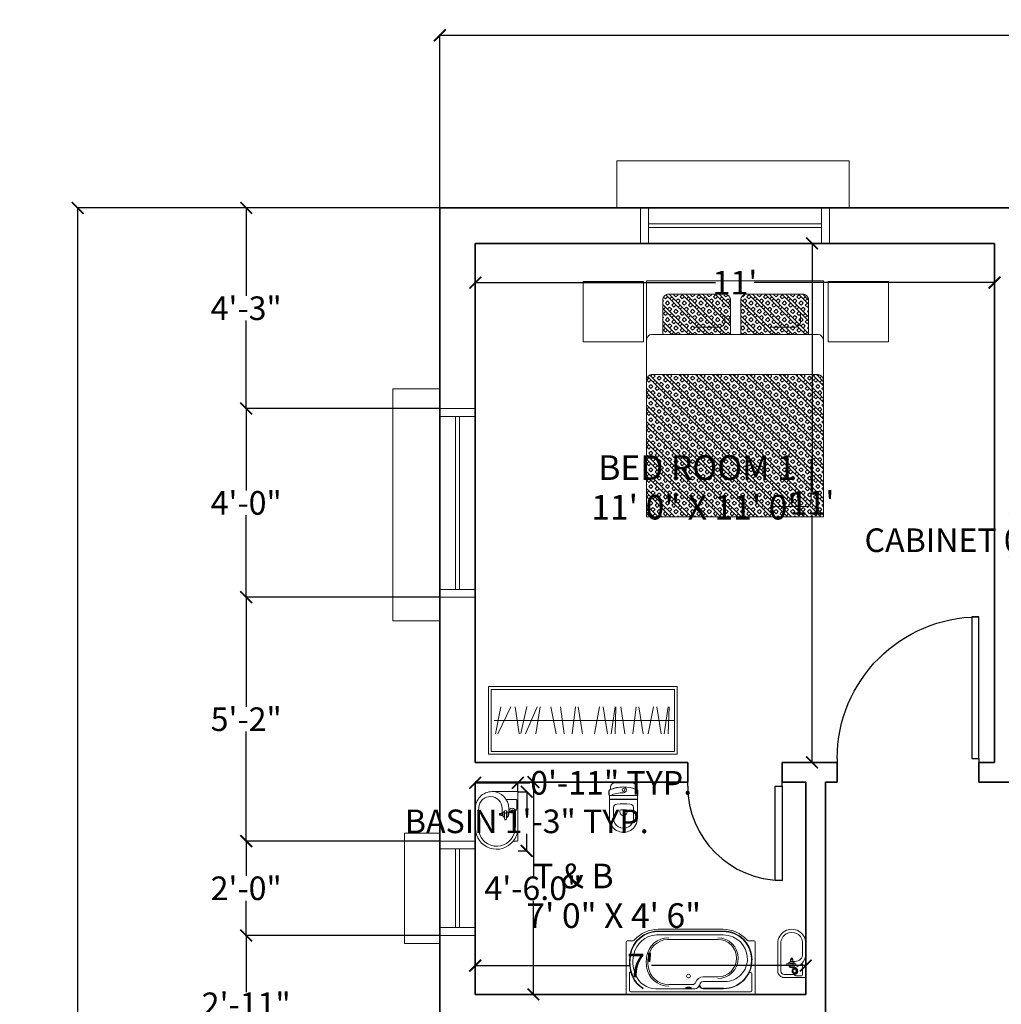
# Model space of a CAD drawing. Units: inches. Extents: x 844 to 2234, y 346 to 1084.
# Tile 49 of 93: x 1590 to 1840, y 828 to 1078. Entities that reach past the tile are written whole.
import ezdxf

# ---------------------------------------------------------------- set-up
doc = ezdxf.new("R2010")
doc.units = ezdxf.units.IN
doc.header["$MEASUREMENT"] = 0
for name, color, linetype, lineweight in [('A-ANNO-DIMS', 2, 'Continuous', 18), ('A-AREA-IDEN', 7, 'Continuous', 18), ('A-FLOR-FIXT', 8, 'Continuous', 18), ('A-WALL', 7, 'Continuous', 35), ('beds', 130, 'Continuous', 18), ('doors', 170, 'Continuous', 25), ('furniture', 8, 'Continuous', 18), ('windows', 1, 'Continuous', 18)]:
    doc.layers.add(name, color=color, linetype=linetype, lineweight=lineweight)
doc.styles.get("Standard").update_dxf_attribs({"font": 'arial.ttf'})
doc.dimstyles.get("Standard").update_dxf_attribs({"dimtxt": 6, "dimasz": 3, "dimexe": 0.18, "dimexo": 0.0625, "dimgap": 0.09, "dimtad": 0, "dimtih": 1, "dimtoh": 1, "dimdec": 1, "dimzin": 0, "dimdsep": 46, "dimlunit": 3, "dimtxsty": 'Standard', "dimblk": 'ARCHTICK', "dimcen": 0.09, "dimadec": 0, "dimazin": 0, "dimtfac": 1, "dimtdec": 1, "dimtofl": 0, "dimtmove": 0, "dimatfit": 3, "dimfxl": 1, "dimtolj": 1, "dimtzin": 0, "dimarcsym": 0})
pattern_1 = [(135, (-1377.70473, -125.71507), (-0.070710678, -0.070710678), []), (135, (-1377.68705, -125.69739), (-0.070710678, -0.070710678), []), (45, (-1377.70473, -125.71507), (-0.070710678, 0.070710678), [-0.025, 0.025]), (45, (-1377.72241, -125.69739), (-0.070710678, 0.070710678), [-0.025, 0.025]), (45, (-1377.74009, -125.67972), (-0.070710678, 0.070710678), [0.025, -0.025]), (45, (-1377.75776, -125.66204), (-0.070710678, 0.070710678), [0.025, -0.025]), (135, (-1377.66938, -125.67972), (-0.070710678, -0.070710678), [0.025, -0.025]), (135, (-1377.6517, -125.66204), (-0.070710678, -0.070710678), [0.025, -0.025])]

# ---------------------------------------------------------------- blocks, each defined once
blk = doc.blocks.new('*U2')
for p, q in [((0, 0), (0, -6)), ((36, 0), (36, -6))]:
    blk.add_line(p, q)
blk.add_lwpolyline([(0, 0), (0, 36), (1.75, 36), (1.75, 0)], close=True)
blk.add_arc((0, 0), 36, 0, 90)
blk = doc.blocks.new('*U4')
for p, q in [((0, 0), (0, -6)), ((24, 0), (24, -6))]:
    blk.add_line(p, q)
blk.add_lwpolyline([(0, 0), (0, 24), (1.75, 24), (1.75, 0)], close=True)
blk.add_arc((0, 0), 24, 0, 90)
blk = doc.blocks.new('MAT-P10')
h = blk.add_hatch()
h.set_pattern_fill('BOX', color=256, scale=0.1, angle=45, style=0)
h.set_pattern_definition(pattern_1)
h.paths.add_polyline_path([(-0.1565, 1.4605), (0.417, 1.4605), (0.417, 1.7513, 0.414214), (0.367, 1.8013), (-0.1065, 1.8013, 0.414214), (-0.1565, 1.7513)])
h.paths.add_polyline_path([(0.5052, 1.4604), (1.0792, 1.4604), (1.0792, 1.7513, 0.414214), (1.0292, 1.8013), (0.5552, 1.8013, 0.414214), (0.5052, 1.7513)])
h = blk.add_hatch()
h.set_pattern_fill('BOX', color=256, scale=0.1, angle=45, style=0)
h.set_pattern_definition(pattern_1)
edge = h.paths.add_edge_path()
edge.add_line((1.2049, -0.085), (1.2049, 1.0625))
edge.add_ellipse((1.1608, 1.0627), major_axis=(0, 0.0568), ratio=0.776379, start_angle=270, end_angle=360)
edge.add_line((1.1608, 1.1195), (-0.251, 1.1195))
edge.add_ellipse((-0.251, 1.0627), major_axis=(0, 0.0568), ratio=0.776379, start_angle=0, end_angle=88.13958)
edge.add_line((-0.2951, 1.0641), (-0.2951, -0.085))
edge.add_line((-0.2951, -0.085), (1.2049, -0.085))
for p, q in [((-0.251, 1.4605), (1.1608, 1.4604)), ((-0.251, 1.1195), (1.1608, 1.1195)), ((1.1017, 0.406), (1.1017, 0.0572)), ((1.0576, 0.0004), (0.7754, 0.0004))]:
    blk.add_line(p, q)
for points in [[(-0.8301, 1.9091), (-0.3191, 1.9091), (-0.3191, 1.3981), (-0.8301, 1.3981)], [(1.2049, -0.085), (-0.2951, -0.085), (-0.2951, 1.9151), (1.2049, 1.915)], [(1.2441, 1.9091), (1.755, 1.9091), (1.755, 1.3981), (1.2441, 1.3981)]]:
    blk.add_lwpolyline(points, close=True)
for points in [[(0.417, 1.4604), (0.417, 1.7513, 0.414214), (0.367, 1.8013), (-0.1065, 1.8013, 0.414214), (-0.1565, 1.7513), (-0.1565, 1.4604)], [(1.0792, 1.4603), (1.0792, 1.7513, 0.414214), (1.0292, 1.8013), (0.5552, 1.8013, 0.414214), (0.5052, 1.7513), (0.5052, 1.4604)], [(0.3702, 1.6242), (0.3702, 1.5715, -0.414214), (0.3202, 1.5215), (0.1113, 1.5215)], [(1.0117, 1.6438), (1.0117, 1.5715, -0.414214), (0.9617, 1.5215), (0.7528, 1.5215)]]:
    blk.add_lwpolyline(points, format="xyb")
at = {"extrusion": (0, 0, -1)}
for centre, start_param, end_param in [((-0.251, 1.4036), 4.712389, 6.283185), ((1.1608, 1.4036), 0, 1.570796), ((-0.251, 1.0627), 4.712389, 6.283185), ((1.1608, 1.0627), 0, 1.570796), ((1.0576, 0.0572), 1.570796, 3.141593), ((1.0576, 0.0572), 1.570796, 3.141593)]:
    blk.add_ellipse(centre, major_axis=(0, 0.0568), ratio=0.776379, start_param=start_param, end_param=end_param, dxfattribs=at)
blk = doc.blocks.new('A$C7A17768A')
for p, q in [((-2.8, 0), (0, 0)), ((-2.8, -1), (-2.8, 0)), ((0, -1), (0, 0)), ((-2.76, -0.04), (-0.04, -0.04)), ((-2.76, -0.96), (-2.76, -0.04)), ((-0.04, -0.96), (-0.04, -0.04)), ((-2.617, -0.3), (-2.694, -0.7)), ((-2.66, -0.7), (-2.466, -0.3)), ((-2.403, -0.3), (-2.342, -0.7)), ((-2.229, -0.296), (-2.317, -0.696)), ((-2.074, -0.3), (-2.25, -0.7)), ((-2.096, -0.7), (-2.033, -0.3)), ((-1.875, -0.3), (-1.796, -0.7)), ((-1.732, -0.3), (-1.675, -0.7)), ((-1.555, -0.7), (-1.507, -0.3)), ((-1.467, -0.3), (-1.403, -0.7)), ((-1.227, -0.7), (-1.151, -0.3)), ((-1.098, -0.3), (-1.034, -0.7)), ((-0.98, -0.7), (-0.921, -0.3)), ((-0.908, -0.3), (-0.919, -0.7)), ((-0.834, -0.3), (-0.777, -0.7)), ((-0.657, -0.7), (-0.61, -0.3)), ((-0.57, -0.3), (-0.505, -0.7)), ((-0.429, -0.7), (-0.353, -0.3)), ((-0.301, -0.3), (-0.237, -0.7)), ((-0.192, -0.7), (-0.133, -0.3)), ((-0.12, -0.3), (-0.131, -0.7)), ((-0.04, -0.5), (-2.716, -0.5)), ((-2.8, -1), (0, -1)), ((-2.76, -0.96), (-0.04, -0.96))]:
    blk.add_line(p, q)
blk = doc.blocks.new('2SABICO')
at = {"color": 0, "linetype": 'ByBlock'}
for p, q in [((0.478, 0.195), (0.089, 0.195)), ((0.478, 0.152), (0.089, 0.152)), ((0, 0.106), (0, 0)), ((0, 0), (0, -0.18)), ((0.043, -0.039), (0.043, 0.106)), ((0.135, 0), (0.135, -0.003)), ((0.168, 0.064), (0.168, -0.015)), ((0.192, 0.064), (0.192, -0.015)), ((0.221, 0.012), (0.222, 0.012)), ((0.223, 0.016), (0.223, -0.016)), ((0.224, 0.017), (0.245, 0.017)), ((0.246, 0.016), (0.246, -0.016)), ((0.25, 0.014), (0.246, 0.014)), ((0.26, 0.01), (0.268, 0.01)), ((0.268, -0.01), (0.268, 0.01)), ((0.268, 0.01), (0.269, 0.009)), ((0.269, -0.009), (0.269, 0.009)), ((0.023, -0.057), (0.023, -0.135)), ((0.135, 0), (0.135, -0.039)), ((0.168, -0.015), (0.192, -0.015)), ((0.168, -0.015), (0.168, -0.046)), ((0.192, -0.015), (0.192, -0.046)), ((0.221, -0.012), (0.222, -0.012)), ((0.224, -0.017), (0.245, -0.017)), ((0.225, -0.017), (0.225, -0.047)), ((0.25, -0.014), (0.246, -0.014)), ((0.26, -0.01), (0.268, -0.01)), ((0.268, -0.01), (0.269, -0.009)), ((0.015, -0.195), (0.478, -0.195)), ((0.038, -0.15), (0.179, -0.15)), ((0.33, -0.152), (0.478, -0.152))]:
    blk.add_line(p, q, dxfattribs=at)
for radius in [0.035, 0.023]:
    blk.add_circle((0.089, -0.039), radius, dxfattribs=at)
for centre, radius, start, end in [((0.089, 0.106), 0.089, 90, 180), ((0.089, 0.106), 0.046, 90, 180), ((0.478, 0), 0.195, 270, 90), ((0.478, 0), 0.152, 270, 90), ((0.18, 0), 0.045, 105.6643, 180), ((0.18, 0), 0.042, 106.8152, 252.6853), ((0.18, 0), 0.0235, 121.1327, 237.8651), ((0.18, 0.064), 0.0121, 0, 180), ((0.18, 0), 0.045, 17.0576, 74.3357), ((0.18, 0), 0.042, 287.3147, 73.1848), ((0.18, 0), 0.0235, 302.1349, 58.8673), ((0.221, 0.013), 0.001, 197.9471, 270), ((0.222, 0.013), 0.001, 270, 0), ((0.224, 0.016), 0.001, 90, 180), ((0.245, 0.016), 0.001, 0, 90), ((0.25, 0), 0.0143, 270, 90), ((0.041, -0.057), 0.018, 99.5941, 180), ((0.038, -0.135), 0.015, 180, 270), ((0.037, -0.033), 0.006, 279.5941, 0), ((0.089, -0.039), 0.046, 180, 360), ((0.326, -0.003), 0.191, 180, 270), ((0.18, -0.046), 0.0125, 180, 0), ((0.179, -0.14), 0.01, 270, 42.9682), ((0.221, -0.013), 0.001, 90, 162.0529), ((0.222, -0.013), 0.001, 0, 90), ((0.224, -0.016), 0.001, 180, 270), ((0.33, -0.047), 0.105, 180, 270), ((0.245, -0.016), 0.001, 270, 0), ((0.015, -0.18), 0.015, 180, 270)]:
    blk.add_arc(centre, radius, start, end, dxfattribs=at)
blk = doc.blocks.new('2SAINCO')
at = {"color": 0, "linetype": 'ByBlock'}
for p, q in [((0.06, 0.181), (0.085, 0.181)), ((0.114, 0.203), (0.165, 0.203)), ((0.496, 0.195), (0.178, 0.195)), ((0.18, -0.188), (0.18, 0.188)), ((0.231, 0.185), (0.231, -0.185)), ((0.234, 0.185), (0.234, -0.185)), ((0.496, 0.14), (0.347, 0.14)), ((0, -0.121), (0, 0.121)), ((0.394, 0.05), (0.407, 0.05)), ((0.394, -0.05), (0.407, -0.05)), ((0.06, -0.181), (0.085, -0.181)), ((0.114, -0.201), (0.165, -0.201)), ((0.114, -0.203), (0.165, -0.203)), ((0.496, -0.195), (0.178, -0.195)), ((0.496, -0.14), (0.347, -0.14))]:
    blk.add_line(p, q, dxfattribs=at)
blk.add_circle((0.1, 0), 0.02, dxfattribs=at)
for centre, radius, start, end in [((0.06, 0.121), 0.06, 90, 180), ((0.517, 0), 0.46, 155.909, 204.091), ((0.085, 0.196), 0.015, 270, 344.534), ((0.114, 0.188), 0.015, 90, 164.534), ((0.165, 0.188), 0.015, 0, 90), ((0.221, 0.185), 0.01, 0, 90), ((0.224, 0.185), 0.01, 0, 90), ((0.347, 0.09), 0.05, 90, 177.3546), ((0.496, 0), 0.195, 270, 90), ((0.496, 0), 0.14, 270, 90), ((0.1, 0), 0.0405, 360, 180), ((0.517, 0), 0.458, 180, 204.67), ((0.66, 0.008), 0.52, 180.891, 201.3823), ((2.295, 0), 2, 177.3546, 182.6454), ((0.677, 0), 0.3, 172.9459, 187.0541), ((0.394, 0.035), 0.015, 90, 172.9459), ((0.407, 0), 0.05, 270, 90), ((0.06, -0.121), 0.06, 180, 270), ((0.347, -0.09), 0.05, 182.6454, 270), ((0.394, -0.035), 0.015, 187.0541, 270), ((0.085, -0.196), 0.015, 15.466, 90), ((0.114, -0.188), 0.015, 195.466, 270), ((0.114, -0.188), 0.013, 195.466, 270), ((0.165, -0.188), 0.013, 270, 30), ((0.165, -0.188), 0.015, 270, 0), ((0.221, -0.185), 0.01, 270, 0), ((0.224, -0.185), 0.01, 270, 0)]:
    blk.add_arc(centre, radius, start, end, dxfattribs=at)
blk = doc.blocks.new('2SABACO')
at = {"color": 0}
for p, q in [((1.341, 0.831), (0.407, 0.831)), ((1.341, 0.91), (0.429, 0.91)), ((1.341, 0.885), (0.429, 0.885)), ((1.341, 0.879), (0.429, 0.879)), ((-0.015, 0.735), (-0.015, 0.015)), ((0, 0.75), (0.08, 0.75)), ((1.263, 0.769), (0.562, 0.769)), ((1.77, 0.75), (1.69, 0.75)), ((1.785, 0.015), (1.785, 0.735)), ((0.03, 0.302), (0.03, 0.053)), ((1.74, 0.053), (1.74, 0.286)), ((0.578, 0.139), (0.911, 0.139)), ((1.263, 0.245), (1.06, 0.245)), ((1.363, 0.181), (1.06, 0.181)), ((0, 0), (1.77, 0)), ((0.048, 0.035), (1.722, 0.035)), ((0.401, 0.08), (0.942, 0.08)), ((1.343, 0.086), (1.06, 0.086)), ((1.343, 0.079), (1.06, 0.079))]:
    blk.add_line(p, q, dxfattribs=at)
blk.add_circle((0.855, 0.256), 0.026, dxfattribs=at)
for centre, radius, start, end in [((0.428, 0.49), 0.395, 98.9726, 181.1954), ((0.428, 0.49), 0.389, 98.9726, 181.2301), ((0.425, 0.49), 0.342, 93.1008, 168.0202), ((0.429, 0.48), 0.43, 90, 139.2943), ((0.429, 0.48), 0.405, 90, 98.9726), ((0.429, 0.48), 0.399, 90, 98.9726), ((1.341, 0.48), 0.43, 40.7057, 90), ((1.341, 0.485), 0.401, 359.4627, 90), ((1.341, 0.485), 0.394, 3.5237, 90), ((1.341, 0.495), 0.336, 0, 90), ((0, 0.735), 0.015, 90, 180), ((0.08, 0.78), 0.03, 270, 319.2943), ((0.578, 0.481), 0.311, 90, 172.609), ((0.578, 0.481), 0.288, 93.3767, 172.609), ((1.263, 0.507), 0.285, 270, 90), ((1.263, 0.507), 0.262, 270, 90), ((1.69, 0.78), 0.03, 220.7057, 270), ((1.77, 0.735), 0.015, 0, 90), ((0.559, 0.454), 0.48, 163.1286, 202.3619), ((0.559, 0.454), 0.528, 177.0415, 202.3619), ((0.559, 0.454), 0.521, 177.0156, 202.3619), ((0.79, 0.454), 0.525, 172.609, 180), ((0.79, 0.454), 0.525, 180, 187.391), ((0.79, 0.454), 0.502, 172.609, 180), ((0.79, 0.454), 0.502, 180, 187.391), ((1.343, 0.477), 0.392, 270, 4.5675), ((1.343, 0.477), 0.398, 270, 0.539), ((1.363, 0.495), 0.314, 270, 2.2815), ((0.042, 0.302), 0.0116, 16.3184, 180.0001), ((0.578, 0.427), 0.311, 187.391, 270), ((0.578, 0.427), 0.288, 187.391, 270), ((1.718, 0.286), 0.0222, 0, 152.9966), ((0.401, 0.389), 0.357, 202.3619, 239.8287), ((0.401, 0.389), 0.351, 202.3619, 239.2093), ((0.401, 0.389), 0.309, 202.3619, 270), ((0.911, 0.183), 0.045, 270, 341.2369), ((1.06, 0.133), 0.112, 90, 161.2369), ((1.06, 0.133), 0.0475, 90, 270), ((0, 0.015), 0.015, 180, 270), ((0.048, 0.053), 0.018, 180, 270), ((0.559, 0.454), 0.48, 250.7818, 251.0555), ((0.821, 0.092), 0.00282, 119.7759, 180), ((0.821, 0.092), 0.00282, 180, 240.2241), ((0.837, 0.064), 0.0347, 103.3326, 119.7759), ((0.835, 0.025), 0.071, 96.5949, 102.1924), ((0.837, 0.12), 0.0347, 240.2241, 256.6674), ((0.847, -0.08), 0.177, 92.7417, 96.5949), ((0.848, 0.02), 0.0808, 95.6065, 103.3326), ((0.848, 0.164), 0.0808, 256.6674, 264.3935), ((0.855, -0.252), 0.349, 90, 92.7417), ((0.855, -0.053), 0.153, 90, 95.6065), ((0.855, 0.237), 0.153, 264.3935, 270), ((0.855, -0.053), 0.153, 84.3935, 90), ((0.855, -0.252), 0.349, 87.2583, 90), ((0.855, 0.237), 0.153, 270, 275.6065), ((0.862, 0.02), 0.0808, 76.6674, 84.3935), ((0.862, 0.164), 0.0808, 275.6065, 283.3326), ((0.863, -0.08), 0.177, 83.4051, 87.2583), ((0.873, 0.064), 0.0347, 60.2241, 76.6674), ((0.873, 0.12), 0.0347, 283.3326, 299.7759), ((0.875, 0.025), 0.071, 77.8076, 83.4051), ((0.889, 0.092), 0.00282, 360, 60.2241), ((0.889, 0.092), 0.00282, 299.7759, 360), ((0.942, 0.145), 0.065, 270, 349.4977), ((1.06, 0.133), 0.054, 180, 270), ((1.722, 0.053), 0.018, 270, 0), ((1.77, 0.015), 0.015, 270, 0)]:
    blk.add_arc(centre, radius, start, end, dxfattribs=at)
blk = doc.blocks.new('2SALACO2')
at = {"color": 0}
for p, q in [((0, 0), (-0.392, 0)), ((0.28, 0), (0, 0)), ((-0.402, -0.01), (-0.402, -0.36)), ((-0.293, -0.026), (-0.293, -0.15)), ((-0.283, -0.016), (-0.166, -0.016)), ((-0.169, -0.128), (-0.085, -0.128)), ((-0.112, -0.035), (-0.133, -0.035)), ((-0.124, -0.035), (0.09, -0.035)), ((0.29, -0.01), (0.29, -0.064)), ((-0.102, -0.219), (-0.169, -0.219)), ((-0.1, -0.161), (-0.131, -0.161)), ((-0.1, -0.186), (-0.131, -0.186)), ((-0.102, -0.217), (-0.102, -0.234)), ((-0.07, -0.216), (-0.101, -0.216)), ((-0.07, -0.235), (-0.101, -0.235)), ((-0.1, -0.161), (-0.1, -0.186)), ((-0.021, -0.161), (-0.1, -0.161)), ((-0.021, -0.186), (-0.1, -0.186)), ((-0.098, -0.214), (-0.098, -0.216)), ((-0.097, -0.239), (-0.098, -0.241)), ((-0.098, -0.241), (-0.098, -0.248)), ((-0.098, -0.241), (-0.073, -0.241)), ((-0.073, -0.248), (-0.098, -0.248)), ((-0.097, -0.235), (-0.097, -0.239)), ((-0.074, -0.239), (-0.097, -0.239)), ((-0.097, -0.248), (-0.097, -0.256)), ((-0.073, -0.256), (-0.097, -0.256)), ((-0.097, -0.256), (-0.094, -0.257)), ((-0.077, -0.257), (-0.094, -0.257)), ((-0.073, -0.256), (-0.077, -0.257)), ((-0.074, -0.235), (-0.074, -0.239)), ((-0.074, -0.239), (-0.073, -0.241)), ((-0.073, -0.214), (-0.073, -0.216)), ((-0.073, -0.241), (-0.073, -0.248)), ((-0.073, -0.248), (-0.073, -0.256)), ((-0.069, -0.217), (-0.069, -0.234))]:
    blk.add_line(p, q, dxfattribs=at)
blk.add_lwpolyline([(-0.402, -0.36, 0.423787), (-0.161, -0.593, 0.423787)], format="xyb", dxfattribs=at)
blk.add_circle((-0.124, -0.081), 0.023, dxfattribs=at)
for centre, radius, start, end in [((-0.392, -0.01), 0.01, 90, 180), ((0.28, -0.01), 0.01, 0, 90), ((-0.169, -0.36), 0.233, 90, 180), ((-0.283, -0.026), 0.01, 90, 180), ((-0.124, -0.081), 0.0462, 90, 270), ((-0.166, -0.046), 0.03, 31.2573, 90), ((-0.133, -0.026), 0.009, 211.2573, 270), ((-0.085, -0.173), 0.042, 16.8152, 162.6853), ((-0.085, -0.173), 0.0458, 15.3964, 90), ((0.09, -0.29), 0.255, 68.9449, 90), ((0.105, -0.295), 0.255, 271.0077, 72.4499), ((0.105, -0.297), 0.297, 271.4871, 51.4524), ((0.105, -0.297), 0.297, 51.4524, 87.1707), ((-0.169, -0.383), 0.164, 90, 265.4963), ((-0.285, -0.15), 0.008, 180, 299.1062), ((-0.131, -0.173), 0.0125, 90, 270), ((-0.085, -0.173), 0.042, 197.3147, 343.1848), ((-0.085, -0.173), 0.0235, 31.1327, 147.8651), ((-0.085, -0.173), 0.0235, 212.1349, 328.8673), ((-0.101, -0.217), 0.001, 90, 180), ((-0.101, -0.234), 0.001, 180, 270), ((-0.085, -0.173), 0.0458, 289.9182, 344.6036), ((-0.07, -0.217), 0.001, 0, 90), ((-0.07, -0.234), 0.001, 270, 0), ((-0.021, -0.173), 0.0121, 270, 90), ((0.021, 4.449), 5, 267.6742, 271.0081), ((-0.017, 4.405), 5, 268.3511, 271.4874)]:
    blk.add_arc(centre, radius, start, end, dxfattribs=at)
blk = doc.blocks.new('_ArchTick')
at = {"color": 0, "linetype": 'ByBlock', "const_width": 0.15}
blk.add_lwpolyline([(-0.5, -0.5), (0.5, 0.5)], dxfattribs=at)
blk = doc.blocks.new('*D88')
at = {"layer": 'A-ANNO-DIMS', "color": 0, "lineweight": -2, "transparency": 16777216}
for p, q in [((1801.84, 1021.46), (1791.52, 1021.46)), ((1791.7, 1021.46), (1791.7, 958.56)), ((1791.7, 889.46), (1791.7, 952.35)), ((1791.16, 889.46), (1791.88, 889.46))]:
    blk.add_line(p, q, dxfattribs=at)
at = {"layer": 'Defpoints', "color": 0, "transparency": 16777216}
for p in [(1801.91, 1021.46), (1791.1, 889.46), (1791.7, 889.46)]:
    blk.add_point(p, dxfattribs=at)
at = {"layer": 'A-ANNO-DIMS', "color": 0, "lineweight": -2, "transparency": 16777216, "xscale": 3, "yscale": 3, "zscale": 3}
for p, rotation in [((1791.7, 1021.46), 90), ((1791.7, 889.46), 270)]:
    blk.add_blockref('_ArchTick', p, dxfattribs=dict(at, rotation=rotation))
at = {"layer": 'A-ANNO-DIMS', "color": 0, "transparency": 16777216, "insert": (1791.7, 955.46), "char_height": 6, "attachment_point": 5}
blk.add_mtext("\\A1;11'", dxfattribs=at)
blk = doc.blocks.new('*D89')
at = {"layer": 'A-ANNO-DIMS', "color": 0, "lineweight": -2, "transparency": 16777216}
for p, q in [((1706.1, 1013.93), (1706.1, 1011.28)), ((1838.1, 1013.93), (1838.1, 1011.28)), ((1706.1, 1011.46), (1767.2, 1011.46)), ((1838.1, 1011.46), (1777, 1011.46))]:
    blk.add_line(p, q, dxfattribs=at)
at = {"layer": 'Defpoints', "color": 0, "transparency": 16777216}
for p in [(1706.1, 1013.99), (1838.1, 1013.99), (1838.1, 1011.46)]:
    blk.add_point(p, dxfattribs=at)
at = {"layer": 'A-ANNO-DIMS', "color": 0, "lineweight": -2, "transparency": 16777216, "xscale": 3, "yscale": 3, "zscale": 3, "rotation": 180}
blk.add_blockref('_ArchTick', (1706.1, 1011.46), dxfattribs=at)
at = {"layer": 'A-ANNO-DIMS', "color": 0, "lineweight": -2, "transparency": 16777216, "xscale": 3, "yscale": 3, "zscale": 3}
blk.add_blockref('_ArchTick', (1838.1, 1011.46), dxfattribs=at)
at = {"layer": 'A-ANNO-DIMS', "color": 0, "transparency": 16777216, "insert": (1772.1, 1011.46), "char_height": 6, "attachment_point": 5}
blk.add_mtext("\\A1;11'", dxfattribs=at)
blk = doc.blocks.new('*D65')
at = {"layer": 'A-ANNO-DIMS', "color": 0, "lineweight": -2, "transparency": 16777216}
for p, q in [((1706.1, 832.65), (1706.1, 837.98)), ((1706.1, 837.8), (1745.27, 837.8)), ((1790.1, 837.8), (1750.93, 837.8)), ((1790.1, 832.65), (1790.1, 837.98))]:
    blk.add_line(p, q, dxfattribs=at)
at = {"layer": 'Defpoints', "color": 0, "transparency": 16777216}
for p in [(1706.1, 837.8), (1706.1, 832.58), (1790.1, 832.58)]:
    blk.add_point(p, dxfattribs=at)
at = {"layer": 'A-ANNO-DIMS', "color": 0, "lineweight": -2, "transparency": 16777216, "xscale": 3, "yscale": 3, "zscale": 3, "rotation": 180}
blk.add_blockref('_ArchTick', (1706.1, 837.8), dxfattribs=at)
at = {"layer": 'A-ANNO-DIMS', "color": 0, "lineweight": -2, "transparency": 16777216, "xscale": 3, "yscale": 3, "zscale": 3}
blk.add_blockref('_ArchTick', (1790.1, 837.8), dxfattribs=at)
at = {"layer": 'A-ANNO-DIMS', "color": 0, "transparency": 16777216, "insert": (1748.1, 837.8), "char_height": 6, "attachment_point": 5}
blk.add_mtext("\\A1;7'", dxfattribs=at)
blk = doc.blocks.new('*D71')
at = {"layer": 'A-ANNO-DIMS', "color": 0, "lineweight": -2, "transparency": 16777216}
for p, q in [((1721.88, 884.46), (1720.68, 884.46)), ((1720.86, 884.46), (1720.86, 860.61)), ((1720.86, 830.46), (1720.86, 854.3)), ((1721.88, 830.46), (1720.68, 830.46))]:
    blk.add_line(p, q, dxfattribs=at)
at = {"layer": 'Defpoints', "color": 0, "transparency": 16777216}
for p in [(1721.94, 884.46), (1720.86, 830.46), (1721.94, 830.46)]:
    blk.add_point(p, dxfattribs=at)
at = {"layer": 'A-ANNO-DIMS', "color": 0, "lineweight": -2, "transparency": 16777216, "xscale": 3, "yscale": 3, "zscale": 3}
for p, rotation in [((1720.86, 884.46), 90), ((1720.86, 830.46), 270)]:
    blk.add_blockref('_ArchTick', p, dxfattribs=dict(at, rotation=rotation))
at = {"layer": 'A-ANNO-DIMS', "color": 0, "transparency": 16777216, "insert": (1720.86, 857.46), "char_height": 6, "attachment_point": 5}
blk.add_mtext('\\A1;4\'-6.0"', dxfattribs=at)
blk = doc.blocks.new('*D86')
at = {"layer": 'A-ANNO-DIMS', "color": 0, "lineweight": -2, "transparency": 16777216}
for p, q in [((1697.1, 1030.52), (1697.1, 1074.57)), ((1697.1, 1074.39), (1920.38, 1074.39)), ((2176.1, 1074.39), (1952.82, 1074.39)), ((2176.1, 1030.52), (2176.1, 1074.57))]:
    blk.add_line(p, q, dxfattribs=at)
at = {"layer": 'Defpoints', "color": 0, "transparency": 16777216}
for p in [(2176.1, 1074.39), (1697.1, 1030.46), (2176.1, 1030.46)]:
    blk.add_point(p, dxfattribs=at)
at = {"layer": 'A-ANNO-DIMS', "color": 0, "lineweight": -2, "transparency": 16777216, "xscale": 3, "yscale": 3, "zscale": 3, "rotation": 180}
blk.add_blockref('_ArchTick', (1697.1, 1074.39), dxfattribs=at)
at = {"layer": 'A-ANNO-DIMS', "color": 0, "lineweight": -2, "transparency": 16777216, "xscale": 3, "yscale": 3, "zscale": 3}
blk.add_blockref('_ArchTick', (2176.1, 1074.39), dxfattribs=at)
at = {"layer": 'A-ANNO-DIMS', "color": 0, "transparency": 16777216, "insert": (1936.6, 1074.39), "char_height": 6, "attachment_point": 5}
blk.add_mtext('\\A1;39\'-11.0"', dxfattribs=at)
blk = doc.blocks.new('*D87')
at = {"layer": 'A-ANNO-DIMS', "color": 0, "lineweight": -2, "transparency": 16777216}
for p, q in [((1697.04, 1030.46), (1604.81, 1030.46)), ((1604.99, 1030.46), (1604.99, 736.11)), ((1604.99, 435.46), (1604.99, 729.8)), ((1697.04, 435.46), (1604.81, 435.46))]:
    blk.add_line(p, q, dxfattribs=at)
at = {"layer": 'Defpoints', "color": 0, "transparency": 16777216}
for p in [(1697.1, 1030.46), (1604.99, 435.46), (1697.1, 435.46)]:
    blk.add_point(p, dxfattribs=at)
at = {"layer": 'A-ANNO-DIMS', "color": 0, "lineweight": -2, "transparency": 16777216, "xscale": 3, "yscale": 3, "zscale": 3}
for p, rotation in [((1604.99, 1030.46), 90), ((1604.99, 435.46), 270)]:
    blk.add_blockref('_ArchTick', p, dxfattribs=dict(at, rotation=rotation))
at = {"layer": 'A-ANNO-DIMS', "color": 0, "transparency": 16777216, "insert": (1604.99, 732.96), "char_height": 6, "attachment_point": 5}
blk.add_mtext('\\A1;49\'-7.0"', dxfattribs=at)
blk = doc.blocks.new('WIN-48IN')
for p, q in [((0, 9), (0, 21)), ((0, 21), (59, 21)), ((59, 9), (59, 21)), ((6, 9), (0, 9)), ((54, 9), (6, 9)), ((6, 9), (6, 0)), ((8, 9), (8, 0)), ((52, 0), (52, 9)), ((54, 0), (54, 9)), ((54, 9), (59, 9)), ((8, 5), (52, 5)), ((8, 4), (52, 4)), ((6, 0), (54, 0))]:
    blk.add_line(p, q)
blk = doc.blocks.new('WIN-24IN')
for p, q in [((9, 28), (0, 28)), ((0, 0), (0, 28)), ((9, 26), (9, 28)), ((18, 26), (9, 26)), ((9, 26), (9, 2)), ((18, 2), (18, 26)), ((18, 24), (9, 24)), ((13, 4), (13, 24)), ((14, 4), (14, 24)), ((9, 4), (18, 4)), ((9, 2), (18, 2)), ((9, 2), (9, 0)), ((9, 0), (0, 0))]:
    blk.add_line(p, q)
blk = doc.blocks.new('*D117')
at = {"layer": 'A-ANNO-DIMS', "color": 0, "lineweight": -2, "transparency": 16777216}
for p, q in [((1716.99, 882.02), (1719.36, 882.02)), ((1719.18, 882.02), (1719.18, 877.68)), ((1719.18, 866.95), (1719.18, 871.29)), ((1716.99, 866.95), (1719.36, 866.95))]:
    blk.add_line(p, q, dxfattribs=at)
at = {"layer": 'Defpoints', "color": 0, "transparency": 16777216}
for p in [(1716.92, 882.02), (1716.92, 866.95), (1719.18, 866.95)]:
    blk.add_point(p, dxfattribs=at)
at = {"layer": 'A-ANNO-DIMS', "color": 0, "lineweight": -2, "transparency": 16777216, "xscale": 3, "yscale": 3, "zscale": 3}
for p, rotation in [((1719.18, 882.02), 90), ((1719.18, 866.95), 270)]:
    blk.add_blockref('_ArchTick', p, dxfattribs=dict(at, rotation=rotation))
at = {"layer": 'A-ANNO-DIMS', "color": 0, "transparency": 16777216, "insert": (1719.18, 874.48), "char_height": 6, "attachment_point": 5}
blk.add_mtext('\\A1;BASIN 1\'-3" TYP.', dxfattribs=at)
blk = doc.blocks.new('*D118')
at = {"layer": 'A-ANNO-DIMS', "color": 0, "lineweight": -2, "transparency": 16777216}
for p, q in [((1706.08, 882.08), (1706.08, 884.46)), ((1706.08, 884.28), (1716.92, 884.28)), ((1716.92, 882.08), (1716.92, 884.46)), ((1716.92, 884.28), (1719.92, 884.28))]:
    blk.add_line(p, q, dxfattribs=at)
at = {"layer": 'Defpoints', "color": 0, "transparency": 16777216}
for p in [(1716.92, 884.28), (1706.08, 882.02), (1716.92, 882.02)]:
    blk.add_point(p, dxfattribs=at)
at = {"layer": 'A-ANNO-DIMS', "color": 0, "lineweight": -2, "transparency": 16777216, "xscale": 3, "yscale": 3, "zscale": 3, "rotation": 180}
blk.add_blockref('_ArchTick', (1706.08, 884.28), dxfattribs=at)
at = {"layer": 'A-ANNO-DIMS', "color": 0, "lineweight": -2, "transparency": 16777216, "xscale": 3, "yscale": 3, "zscale": 3}
blk.add_blockref('_ArchTick', (1716.92, 884.28), dxfattribs=at)
at = {"layer": 'A-ANNO-DIMS', "color": 0, "transparency": 16777216, "insert": (1740.63, 884.28), "char_height": 6, "attachment_point": 5}
blk.add_mtext('\\A1;0\'-11" TYP.', dxfattribs=at)
blk = doc.blocks.new('*D127')
at = {"layer": 'A-ANNO-DIMS', "color": 0, "lineweight": -2, "transparency": 16777216}
for p, q in [((1844.9, 951.36), (1843.17, 951.36)), ((1843.35, 951.36), (1843.35, 949.16)), ((1843.35, 940.57), (1843.35, 942.78)), ((1844.9, 940.57), (1843.17, 940.57))]:
    blk.add_line(p, q, dxfattribs=at)
at = {"layer": 'Defpoints', "color": 0, "transparency": 16777216}
for p in [(1843.35, 951.36), (1844.97, 951.36), (1844.97, 940.57)]:
    blk.add_point(p, dxfattribs=at)
at = {"layer": 'A-ANNO-DIMS', "color": 0, "lineweight": -2, "transparency": 16777216, "xscale": 3, "yscale": 3, "zscale": 3}
for p, rotation in [((1843.35, 951.36), 90), ((1843.35, 940.57), 270)]:
    blk.add_blockref('_ArchTick', p, dxfattribs=dict(at, rotation=rotation))
at = {"layer": 'A-ANNO-DIMS', "color": 0, "transparency": 16777216, "insert": (1843.35, 945.97), "char_height": 6, "attachment_point": 5}
blk.add_mtext('\\A1;CABINET 0\'-11" TYP.', dxfattribs=at)
blk = doc.blocks.new('*D167')
at = {"layer": 'A-ANNO-DIMS', "color": 0, "lineweight": -2, "transparency": 16777216}
for p, q in [((1697.04, 845.46), (1647.67, 845.46)), ((1647.85, 845.46), (1647.85, 831.06)), ((1647.85, 810.46), (1647.85, 824.85)), ((1697.04, 810.46), (1647.67, 810.46))]:
    blk.add_line(p, q, dxfattribs=at)
at = {"layer": 'Defpoints', "color": 0, "transparency": 16777216}
for p in [(1647.85, 845.46), (1697.1, 845.46), (1697.1, 810.46)]:
    blk.add_point(p, dxfattribs=at)
at = {"layer": 'A-ANNO-DIMS', "color": 0, "lineweight": -2, "transparency": 16777216, "xscale": 3, "yscale": 3, "zscale": 3}
for p, rotation in [((1647.85, 845.46), 90), ((1647.85, 810.46), 270)]:
    blk.add_blockref('_ArchTick', p, dxfattribs=dict(at, rotation=rotation))
at = {"layer": 'A-ANNO-DIMS', "color": 0, "transparency": 16777216, "insert": (1647.85, 827.96), "char_height": 6, "attachment_point": 5}
blk.add_mtext('\\A1;2\'-11"', dxfattribs=at)
blk = doc.blocks.new('*D168')
at = {"layer": 'A-ANNO-DIMS', "color": 0, "lineweight": -2, "transparency": 16777216}
for p, q in [((1697.04, 869.46), (1647.67, 869.46)), ((1647.85, 869.46), (1647.85, 860.61)), ((1647.85, 845.46), (1647.85, 854.3)), ((1697.04, 845.46), (1647.67, 845.46))]:
    blk.add_line(p, q, dxfattribs=at)
at = {"layer": 'Defpoints', "color": 0, "transparency": 16777216}
for p in [(1647.85, 869.46), (1697.1, 869.46), (1697.1, 845.46)]:
    blk.add_point(p, dxfattribs=at)
at = {"layer": 'A-ANNO-DIMS', "color": 0, "lineweight": -2, "transparency": 16777216, "xscale": 3, "yscale": 3, "zscale": 3}
for p, rotation in [((1647.85, 869.46), 90), ((1647.85, 845.46), 270)]:
    blk.add_blockref('_ArchTick', p, dxfattribs=dict(at, rotation=rotation))
at = {"layer": 'A-ANNO-DIMS', "color": 0, "transparency": 16777216, "insert": (1647.85, 857.46), "char_height": 6, "attachment_point": 5}
blk.add_mtext('\\A1;2\'-0"', dxfattribs=at)
blk = doc.blocks.new('*D169')
at = {"layer": 'A-ANNO-DIMS', "color": 0, "lineweight": -2, "transparency": 16777216}
for p, q in [((1697.04, 931.46), (1647.67, 931.46)), ((1647.85, 931.46), (1647.85, 903.61)), ((1647.85, 869.46), (1647.85, 897.3)), ((1697.04, 869.46), (1647.67, 869.46))]:
    blk.add_line(p, q, dxfattribs=at)
at = {"layer": 'Defpoints', "color": 0, "transparency": 16777216}
for p in [(1647.85, 931.46), (1697.1, 931.46), (1697.1, 869.46)]:
    blk.add_point(p, dxfattribs=at)
at = {"layer": 'A-ANNO-DIMS', "color": 0, "lineweight": -2, "transparency": 16777216, "xscale": 3, "yscale": 3, "zscale": 3}
for p, rotation in [((1647.85, 931.46), 90), ((1647.85, 869.46), 270)]:
    blk.add_blockref('_ArchTick', p, dxfattribs=dict(at, rotation=rotation))
at = {"layer": 'A-ANNO-DIMS', "color": 0, "transparency": 16777216, "insert": (1647.85, 900.46), "char_height": 6, "attachment_point": 5}
blk.add_mtext('\\A1;5\'-2"', dxfattribs=at)
blk = doc.blocks.new('*D170')
at = {"layer": 'A-ANNO-DIMS', "color": 0, "lineweight": -2, "transparency": 16777216}
for p, q in [((1697.04, 979.46), (1647.67, 979.46)), ((1647.85, 979.46), (1647.85, 958.61)), ((1647.85, 931.46), (1647.85, 952.3)), ((1697.04, 931.46), (1647.67, 931.46))]:
    blk.add_line(p, q, dxfattribs=at)
at = {"layer": 'Defpoints', "color": 0, "transparency": 16777216}
for p in [(1647.85, 979.46), (1697.1, 979.46), (1697.1, 931.46)]:
    blk.add_point(p, dxfattribs=at)
at = {"layer": 'A-ANNO-DIMS', "color": 0, "lineweight": -2, "transparency": 16777216, "xscale": 3, "yscale": 3, "zscale": 3}
for p, rotation in [((1647.85, 979.46), 90), ((1647.85, 931.46), 270)]:
    blk.add_blockref('_ArchTick', p, dxfattribs=dict(at, rotation=rotation))
at = {"layer": 'A-ANNO-DIMS', "color": 0, "transparency": 16777216, "insert": (1647.85, 955.46), "char_height": 6, "attachment_point": 5}
blk.add_mtext('\\A1;4\'-0"', dxfattribs=at)
blk = doc.blocks.new('*D171')
at = {"layer": 'A-ANNO-DIMS', "color": 0, "lineweight": -2, "transparency": 16777216}
for p, q in [((1697.04, 1030.46), (1647.67, 1030.46)), ((1647.85, 1030.46), (1647.85, 1008.11)), ((1647.85, 979.46), (1647.85, 1001.8)), ((1697.04, 979.46), (1647.67, 979.46))]:
    blk.add_line(p, q, dxfattribs=at)
at = {"layer": 'Defpoints', "color": 0, "transparency": 16777216}
for p in [(1647.85, 1030.46), (1697.1, 1030.46), (1697.1, 979.46)]:
    blk.add_point(p, dxfattribs=at)
at = {"layer": 'A-ANNO-DIMS', "color": 0, "lineweight": -2, "transparency": 16777216, "xscale": 3, "yscale": 3, "zscale": 3}
for p, rotation in [((1647.85, 1030.46), 90), ((1647.85, 979.46), 270)]:
    blk.add_blockref('_ArchTick', p, dxfattribs=dict(at, rotation=rotation))
at = {"layer": 'A-ANNO-DIMS', "color": 0, "transparency": 16777216, "insert": (1647.85, 1004.96), "char_height": 6, "attachment_point": 5}
blk.add_mtext('\\A1;4\'-3"', dxfattribs=at)

msp = doc.modelspace()

# ---------------------------------------------------------------- linework, layer by layer
at = {"layer": 'A-WALL'}
for p, q in [((1697.1, 1030.46), (1697.1, 435.46)), ((1697.1, 1030.46), (2176.1, 1030.46)), ((1706.1, 1021.46), (1706.1, 889.46)), ((1706.1, 1021.46), (1838.1, 1021.46)), ((1838.1, 1021.46), (1838.1, 889.46)), ((1706.1, 889.46), (1760.1, 889.46)), ((1760.1, 884.46), (1760.1, 889.46)), ((1784.1, 889.46), (1798.1, 889.46)), ((1784.1, 884.46), (1784.1, 889.46)), ((1798.1, 889.46), (1798.1, 884.46)), ((1834.1, 889.46), (1838.1, 889.46)), ((1834.1, 889.46), (1834.1, 884.46)), ((1706.1, 884.46), (1706.1, 830.46)), ((1706.1, 884.46), (1760.1, 884.46)), ((1784.1, 884.46), (1790.1, 884.46)), ((1790.1, 884.46), (1790.1, 830.46)), ((1795.1, 884.46), (1795.1, 795.46)), ((1795.1, 884.46), (1798.1, 884.46)), ((1834.1, 884.46), (1886.1, 884.46)), ((1706.1, 830.46), (1790.1, 830.46))]:
    msp.add_line(p, q, dxfattribs=at)

# ---------------------------------------------------------------- block references
at = {"layer": 'A-FLOR-FIXT', "xscale": 18.21101258924898, "yscale": 18.21101258924898, "zscale": 18.21101258924898}
for name, p, rotation in [('2SAINCO', (1743.76, 884.29), 270), ('2SALACO2', (1716.92, 874.71), 270), ('2SABICO', (1786.55, 834.78), 89.99999999999999)]:
    msp.add_blockref(name, p, dxfattribs=dict(at, rotation=rotation))
msp.add_blockref('2SABACO', (1744.73, 830.46), dxfattribs=at)
at = {"layer": 'beds', "xscale": 29.99962925113936, "yscale": 29.99962925113936, "zscale": 29.99962925113936}
msp.add_blockref('MAT-P10', (1758.45, 954.49), dxfattribs=at)
at = {"layer": 'doors', "xscale": -1}
msp.add_blockref('*U2', (1834.1, 890.46), dxfattribs=at)
at = {"layer": 'doors', "rotation": 180}
msp.add_blockref('*U4', (1784.1, 883.46), dxfattribs=at)
at = {"layer": 'furniture', "xscale": 17.14285714285603, "yscale": 17.14285714285603, "zscale": 17.14285714285603}
msp.add_blockref('A$C7A17768A', (1757.41, 908.73), dxfattribs=at)
at = {"layer": 'windows'}
for name, p in [('WIN-48IN', (1742.1, 1021.46)), ('WIN-24IN', (1688.1, 843.46))]:
    msp.add_blockref(name, p, dxfattribs=at)
at = {"layer": 'windows', "rotation": 90.00000000000175}
msp.add_blockref('WIN-48IN', (1706.1, 925.46), dxfattribs=at)

# ---------------------------------------------------------------- texts
at = {"layer": 'A-AREA-IDEN'}
for s, height, p in [('BED ROOM 1', 6.269, (1737.37, 961.3)), (' 11\' 0" X 11\' 0"', 6.2688, (1733.67, 951.23)), ('T & B', 6.269, (1720.86, 857.46)), (' 7\' 0" X 4\' 6"', 6.2688, (1717.17, 847.38))]:
    msp.add_text(s, height=height, dxfattribs=at).set_placement(p)

# ---------------------------------------------------------------- dimensions: what is measured, and where the dimension line sits
at = {"layer": 'A-ANNO-DIMS'}
for base, p1, p2, picture, middle in [((2176.1, 1074.39), (1697.1, 1030.46), (2176.1, 1030.46), '*D86', (1936.6, 1074.39)), ((1838.1, 1011.46), (1706.1, 1013.99), (1838.1, 1013.99), '*D89', (1772.1, 1011.46)), ((1706.1, 837.8), (1790.1, 832.58), (1706.1, 832.58), '*D65', (1748.1, 837.8))]:
    dim = msp.add_linear_dim(base=base, p1=p1, p2=p2, dimstyle='Standard', override={"dimclrd": 0, "dimclre": 0, "dimclrt": 0}, dxfattribs=at)
    dim.commit()
    dim.dimension.update_dxf_attribs({"geometry": picture, "text_midpoint": middle})
for base, p1, p2, override, picture, middle in [((1604.99, 435.46), (1697.1, 1030.46), (1697.1, 435.46), {"dimclrd": 0, "dimclre": 0, "dimclrt": 0}, '*D87', (1604.99, 732.96)), ((1647.85, 1030.46), (1697.1, 979.46), (1697.1, 1030.46), {"dimdec": 1, "dimlfac": 1, "dimrnd": 0, "dimzin": 1, "dimdsep": 46, "dimlunit": 4, "dimfrac": 2}, '*D171', (1647.85, 1004.96)), ((1791.7, 889.46), (1801.91, 1021.46), (1791.1, 889.46), {"dimclrd": 0, "dimclre": 0, "dimclrt": 0}, '*D88', (1791.7, 955.46)), ((1647.85, 979.46), (1697.1, 931.46), (1697.1, 979.46), {"dimdec": 1, "dimlfac": 1, "dimrnd": 0, "dimzin": 1, "dimdsep": 46, "dimlunit": 4, "dimfrac": 2}, '*D170', (1647.85, 955.46)), ((1647.85, 931.46), (1697.1, 869.46), (1697.1, 931.46), {"dimdec": 1, "dimlfac": 1, "dimrnd": 0, "dimzin": 1, "dimdsep": 46, "dimlunit": 4, "dimfrac": 2}, '*D169', (1647.85, 900.46)), ((1720.86, 830.46), (1721.94, 884.46), (1721.94, 830.46), {"dimclrd": 0, "dimclre": 0, "dimclrt": 0}, '*D71', (1720.86, 857.46)), ((1647.85, 869.46), (1697.1, 845.46), (1697.1, 869.46), {"dimdec": 1, "dimlfac": 1, "dimrnd": 0, "dimzin": 1, "dimdsep": 46, "dimlunit": 4, "dimfrac": 2}, '*D168', (1647.85, 857.46)), ((1647.85, 845.46), (1697.1, 810.46), (1697.1, 845.46), {"dimdec": 1, "dimlfac": 1, "dimrnd": 0, "dimzin": 1, "dimdsep": 46, "dimlunit": 4, "dimfrac": 2}, '*D167', (1647.85, 827.96))]:
    dim = msp.add_linear_dim(base=base, p1=p1, p2=p2, angle=90, dimstyle='Standard', override=override, dxfattribs=at)
    dim.commit()
    dim.dimension.update_dxf_attribs({"geometry": picture, "text_midpoint": middle})
for base, p1, p2, angle, text, picture, middle in [((1843.35, 951.36), (1844.97, 940.57), (1844.97, 951.36), 90, 'CABINET <> TYP.', '*D127', (1843.35, 945.97)), ((1719.18, 866.95), (1716.92, 882.02), (1716.92, 866.95), 270, 'BASIN <> TYP.', '*D117', (1719.18, 874.48))]:
    dim = msp.add_linear_dim(base=base, p1=p1, p2=p2, angle=angle, text=text, dimstyle='Standard', override={"dimdec": 1, "dimlfac": 1, "dimrnd": 0, "dimzin": 1, "dimdsep": 46, "dimlunit": 4, "dimfrac": 2}, dxfattribs=at)
    dim.commit()
    dim.dimension.update_dxf_attribs({"geometry": picture, "text_midpoint": middle})
dim = msp.add_linear_dim(base=(1716.92, 884.28), p1=(1706.08, 882.02), p2=(1716.92, 882.02), text='<> TYP.', dimstyle='Standard', override={"dimdec": 1, "dimlfac": 1, "dimrnd": 0, "dimzin": 1, "dimdsep": 46, "dimlunit": 4, "dimfrac": 2}, dxfattribs=at)
dim.commit()
dim.dimension.update_dxf_attribs({"geometry": '*D118', "text_midpoint": (1740.63, 884.28)})

doc.saveas('drawing.dxf')
